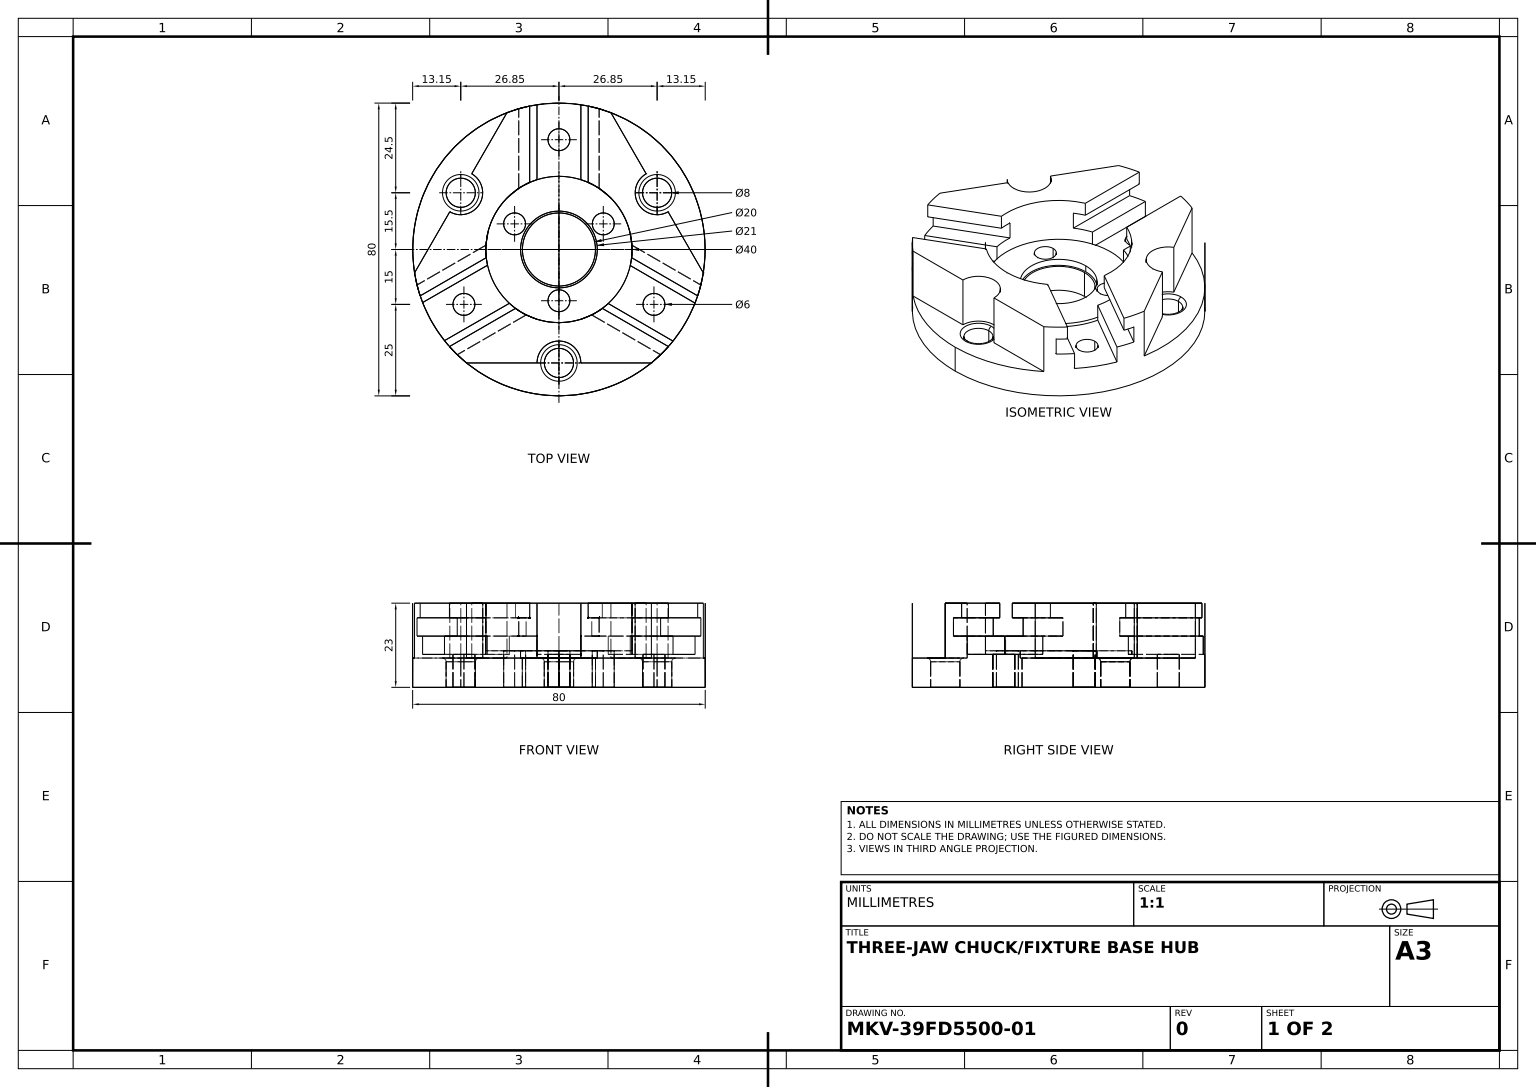
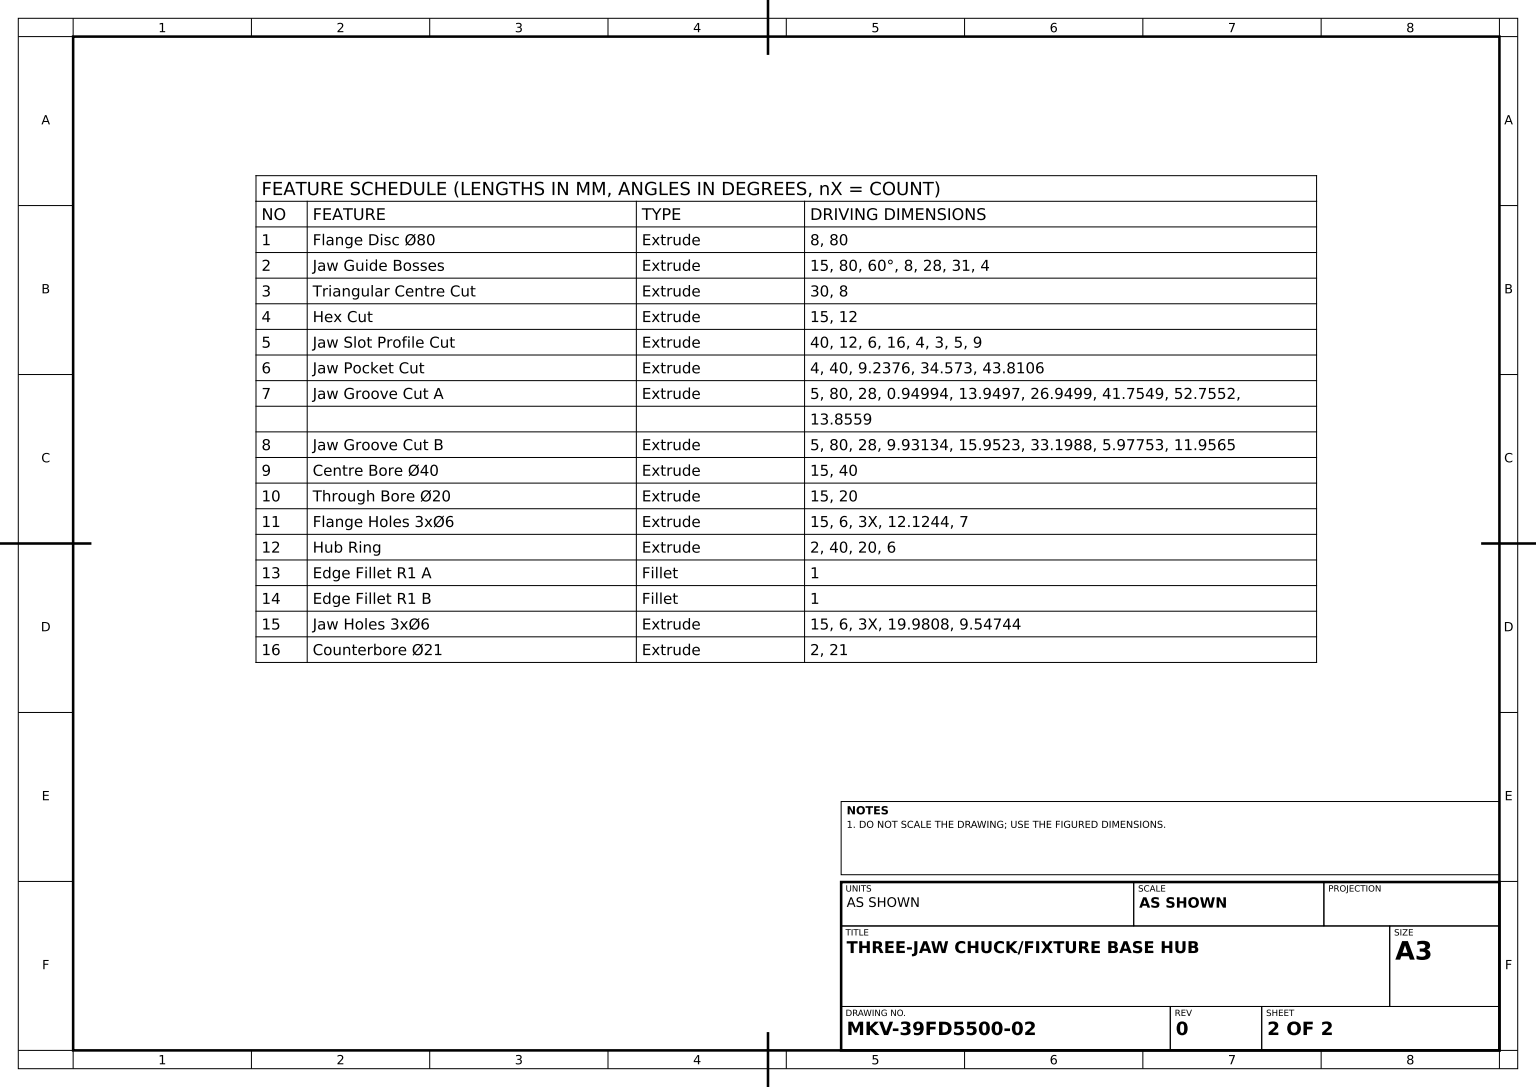
SolidWorks part; units mm, degrees
material "Plain Carbon Steel"
ref_plane "Front Plane" through (0, 0, 0) normal (0, 0, 1) x (1, 0, 0)
ref_plane "Top Plane" through (0, 0, 0) normal (0, 1, 0) x (1, 0, 0)
ref_plane "Right Plane" through (0, 0, 0) normal (1, 0, 0) x (0, 0, -1)
sketch "Flange Disc Sketch" plane through (0, 0, 0) normal (0, 1, 0) x (1, 0, 0)
  circle A0 centre (0, 0) radius 40
  dimension "D1" = 80
extrude "Flange Disc Ø80" add sketch "Flange Disc Sketch" along normal blind 8
sketch "Jaw Guide Bosses Sketch" plane through (0, 8, 0) normal (0, 1, 0) x (1, 0, 0)
  line L0 (-28.8468, 12.0359) -> (-39.486, -6.3918)
  line L1 (31, -31) -> (4, -31)
  line L2 (-14.2076, 37.3918) -> (-24.8468, 18.9641)
  line L3 (14.2076, 37.3918) -> (24.8468, 18.9641)
  line L4 (28.8468, 12.0359) -> (39.486, -6.3918)
  line L5 (-4, -31) -> (-25.2784, -31)
  arc A1 (14.2076, 37.3918) -> (-14.2076, 37.3918) centre (0, 0) ccw
  arc A2 (-39.486, -6.3918) -> (-25.2784, -31) centre (0, 0) ccw
  arc A3 (25.2784, -31) -> (39.486, -6.3918) centre (0, 0) ccw
  circle A4 centre (-26.8468, 15.5) radius 4
  circle A5 centre (0, -31) radius 4
  circle A6 centre (26.8468, 15.5) radius 4
  circle A8 centre (0, 0) radius 14
  circle A9 centre (0, 0) radius 40 construction
  circle M4 centre (0, 0) radius 40
  dimension "D1" = 4
  dimension "D2" = 80
  dimension "D5" = 8
  dimension "D6" = 8
  dimension "D7" = 8
  dimension "D8" = 28
  dimension "D3" = 60
  dimension "D4" = 60
  dimension "D9" = 31
  dimension "D10" = 31
extrude "Jaw Guide Bosses" add sketch "Jaw Guide Bosses Sketch" along normal blind 15 contours A6 L3 L2 A4 L0 L5 A5 L1 L4 A8 M4
sketch "Triangular Centre Cut Sketch" plane through (0, 23, 0) normal (0, 1, 0) x (1, 0, 0)
  circle A0 centre (-26.8468, 15.5) radius 4
  circle A1 centre (26.8468, 15.5) radius 4
  circle A2 centre (0, -31) radius 4
  dimension "D1" = 8
  dimension "D2" = 8
  dimension "D3" = 8
extrude "Triangular Centre Cut" cut sketch "Triangular Centre Cut Sketch" against normal blind 30
sketch "Hex Cut Sketch" plane through (0, 23, 0) normal (0, 1, 0) x (1, 0, 0)
  line L0 (-29.8468, 10.3038) -> (-23.8468, 20.6962)
  line L1 (-28.8468, 12.0359) -> (-39.486, -6.3918) construction
  line L2 (-14.2076, 37.3918) -> (-24.8468, 18.9641) construction
  line L3 (23.8468, 20.6962) -> (29.8468, 10.3038)
  line L4 (14.2076, 37.3918) -> (24.8468, 18.9641) construction
  line L5 (28.8468, 12.0359) -> (39.486, -6.3918) construction
  line L6 (-6, -31) -> (6, -31)
  arc A0 (-29.8468, 10.3038) -> (-23.8468, 20.6962) centre (-26.8468, 15.5) ccw
  arc A1 (23.8468, 20.6962) -> (29.8468, 10.3038) centre (26.8468, 15.5) ccw
  arc A2 (6, -31) -> (-6, -31) centre (0, -31) ccw
  dimension "D1" = 12
  dimension "D2" = 12
  dimension "D3" = 12
extrude "Hex Cut" cut sketch "Hex Cut Sketch" against normal blind 15
ref_plane "Plane1" through (0, 0, -40) normal (0, 0, 1) x (1, 0, 0)
sketch "Jaw Slot Profile Sketch" plane through (0, 0, -40) normal (0, 0, 1) x (1, 0, 0)
  line L1 (8, 23) -> (-8, 23)
  line L2 (-6, 9) -> (6, 9)
  line L4 (14.2076, 23) -> (-14.2076, 23) construction
  line L6 (8, 23) -> (8, 19)
  line L7 (8, 19) -> (11, 19)
  line L8 (11, 19) -> (11, 14)
  line L9 (11, 14) -> (6, 14)
  line L10 (6, 14) -> (6, 9)
  line L14 (-6, 14) -> (-6, 9)
  line L15 (-11, 14) -> (-6, 14)
  line L16 (-11, 19) -> (-11, 14)
  line L17 (-8, 19) -> (-11, 19)
  line L18 (-8, 23) -> (-8, 19)
  point P7 (0, 23)
  dimension "D1" = 12
  dimension "D2" = 6
  dimension "D3" = 16
  dimension "D4" = 4
  dimension "D5" = 3
  dimension "D6" = 5
  dimension "D7" = 5
  dimension "D8" = 9
  dimension "D9" = 5
  dimension "D10" = 4
  dimension "D11" = 5
  dimension "D12" = 5
  dimension "D13" = 5
extrude "Jaw Slot Profile Cut" cut sketch "Jaw Slot Profile Sketch" along normal blind 40
sketch "Jaw Pocket Sketch" plane through (0, 23, 0) normal (0, 1, 0) x (1, 0, 0)
  line L2 (0, 9.2376) -> (37.9411, -12.6677)
  line L3 (0, 9.2376) -> (-37.9411, -12.6677)
  line L4 (0, -9.2376) -> (29.9411, -26.5241)
  line L5 (0, -9.2376) -> (-29.9411, -26.5241)
  arc A0 (-39.486, -6.3918) -> (-25.2784, -31) centre (0, 0) ccw construction
  arc A1 (25.2784, -31) -> (39.486, -6.3918) centre (0, 0) ccw construction
  arc A2 (-37.9411, -12.6677) -> (-29.9411, -26.5241) centre (0, 0) ccw
  arc A3 (37.9411, -12.6677) -> (29.9411, -26.5241) centre (0, 0) cw
  point P11 (38.641, -13.0718)
  point P12 (-38.641, -13.0718)
  point P14 (30.641, -26.9282)
  point P15 (-30.641, -26.9282)
  dimension "D3" = 40
  dimension "D4" = 40
  dimension "D1" = 9.2376
  dimension "D2" = 9.2376
  dimension "D5" = 34.573
  dimension "D6" = 43.8106
extrude "Jaw Pocket Cut" cut sketch "Jaw Pocket Sketch" against normal blind 4
sketch "Jaw Groove Sketch A" plane through (0, 19, 0) normal (0, 1, 0) x (1, 0, 0)
  line L2 (13.0001, 5.196) -> (38.8053, -9.7031)
  line L3 (-12.9999, 5.1963) -> (-38.8055, -9.7021)
  line L4 (-0.0002, -12.7017) -> (27.805, -28.7555)
  line L5 (-0.0002, -12.7017) -> (-27.8058, -28.7548)
  arc A0 (-38.8055, -9.7021) -> (-27.8058, -28.7548) centre (0, 0) ccw
  arc A1 (-12.9999, 5.1963) -> (13.0001, 5.196) centre (0, 0) ccw
  arc A2 (27.805, -28.7555) -> (38.8053, -9.7031) centre (0, 0) ccw
  point P1 (-62.9273, -36.33)
  point P2 (0.0002, 12.7017)
  point P3 (58.6667, -21.1704)
  point P4 (53.1666, -30.6967)
  point P6 (-68.4272, -26.8037)
  point P8 (47.6665, -40.2229)
  point P9 (-57.4274, -45.8564)
  line M3 (-13.9499, 1.1836) -> (-37.9411, -12.6677)
  arc M4 (-37.9411, -12.6677) -> (-29.9411, -26.5241) centre (0, 0) ccw
  line M5 (-29.9411, -26.5241) -> (-5.9499, -12.6728)
  arc M6 (-5.9499, -12.6728) -> (-13.9499, 1.1836) centre (0, 0) cw
  dimension "D1" = 0.9499
  dimension "D4" = 80
  dimension "D5" = 28
  dimension "D2" = 13.9497
  dimension "D3" = 26.9499
  dimension "D6" = 41.7549
  dimension "D7" = 52.7552
  dimension "D8" = 13.8559
extrude "Jaw Groove Cut A" cut sketch "Jaw Groove Sketch A" against normal blind 5 contours A1 A0 L5 M5 | A1 L3 A0 M3 | M6 M3 M4 M5 | L4 A2 L2 A1
sketch "Jaw Groove Sketch B" plane through (0, 14, 0) normal (0, 1, 0) x (1, 0, 0)
  line L2 (13.9521, -1.1566) -> (37.2196, -14.6528)
  line L3 (-13.9567, -1.1002) -> (-37.2785, -14.5023)
  line L4 (7.9312, -11.5368) -> (31.1986, -25.0329)
  line L5 (-7.9777, -11.5046) -> (-31.2995, -24.9067)
  arc A0 (-37.2785, -14.5023) -> (-31.2995, -24.9067) centre (0, 0) ccw
  arc A1 (-13.9567, -1.1002) -> (-7.9777, -11.5046) centre (0, 0) ccw
  arc A2 (31.1986, -25.0329) -> (37.2196, -14.6528) centre (0, 0) ccw
  arc A3 (7.9312, -11.5368) -> (13.9521, -1.1566) centre (0, 0) ccw
  point P1 (-53.5057, -30.7476)
  point P3 (0.014, 6.9282)
  point P4 (52.921, -30.6967)
  point P6 (-56.4952, -25.5454)
  point P7 (-0.014, -6.9282)
  point P9 (-50.5162, -35.9498)
  dimension "D4" = 80
  dimension "D5" = 28
  dimension "D1" = 9.9313
  dimension "D2" = 15.9523
  dimension "D3" = 33.1988
  dimension "D6" = 5.9775
  dimension "D7" = 11.9565
extrude "Jaw Groove Cut B" cut sketch "Jaw Groove Sketch B" against normal blind 5
sketch "Centre Bore Sketch" plane through (0, 23, 0) normal (0, 1, 0) x (1, 0, 0)
  circle A0 centre (0, 0) radius 20
  dimension "D1" = 40
extrude "Centre Bore Ø40" cut sketch "Centre Bore Sketch" against normal blind 15
sketch "Through Bore Sketch" plane through (0, 8, 0) normal (0, 1, 0) x (1, 0, 0)
  circle A0 centre (0, 0) radius 10
  dimension "D1" = 20
extrude "Through Bore Ø20" cut sketch "Through Bore Sketch" against normal blind 15
sketch "Flange Holes Sketch" plane through (0, 8, 0) normal (0, 1, 0) x (1, 0, 0)
  circle A1 centre (0, -14) radius 3
  circle A2 centre (-12.1244, 7) radius 3
  circle A3 centre (12.1244, 7) radius 3
  circle A4 centre (0, 0) radius 10 construction
  dimension "D1" = 6
  dimension "D3" = 12.1244
  dimension "D4" = 12.1244
  dimension "D5" = 7
  dimension "D2" = 3
extrude "Flange Holes 3xØ6" cut sketch "Flange Holes Sketch" against normal blind 15
sketch "Hub Ring Sketch" plane through (0, 8, 0) normal (0, 1, 0) x (1, 0, 0)
  circle A1 centre (0, 0) radius 10
  circle A2 centre (0, 0) radius 20
  circle A3 centre (-12.1244, 7) radius 3
  circle A4 centre (12.1244, 7) radius 3
  circle A5 centre (0, -14) radius 3
  dimension "D1" = 40
  dimension "D2" = 20
  dimension "D3" = 6
  dimension "D4" = 6
  dimension "D5" = 6
extrude "Hub Ring" add sketch "Hub Ring Sketch" along normal blind 2
fillet "Edge Fillet R1 A" radius 1 1 edges at (26.8468, 8, -11.5)
fillet "Edge Fillet R1 B" radius 1 2 edges at (0, 8, 35) (-26.8468, 8, -11.5)
sketch "Jaw Holes Sketch" plane through (0, 9, 0) normal (0, 1, 0) x (1, 0, 0)
  line L0 (6, 19.0788) -> (6, 39.5474) construction
  circle A1 centre (0, 30) radius 3
  circle A2 centre (25.9808, -15) radius 3
  circle A3 centre (-25.9808, -15) radius 3
  dimension "D1" = 6
  dimension "D3" = 19.9808
  dimension "D4" = 6
  dimension "D5" = 9.5474
  dimension "D2" = 3
extrude "Jaw Holes 3xØ6" cut sketch "Jaw Holes Sketch" against normal blind 15
sketch "Counterbore Sketch" plane through (0, 10, 0) normal (0, 1, 0) x (1, 0, 0)
  circle A0 centre (0, 0) radius 10.5
  dimension "D1" = 21
extrude "Counterbore Ø21" cut sketch "Counterbore Sketch" against normal blind 2
